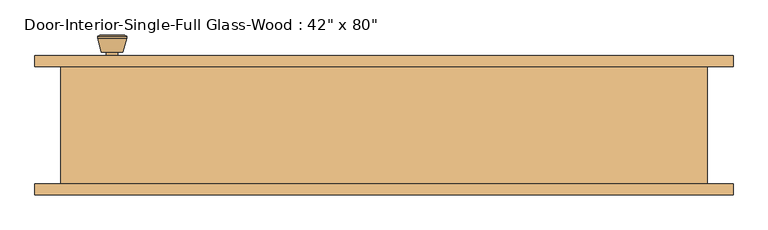
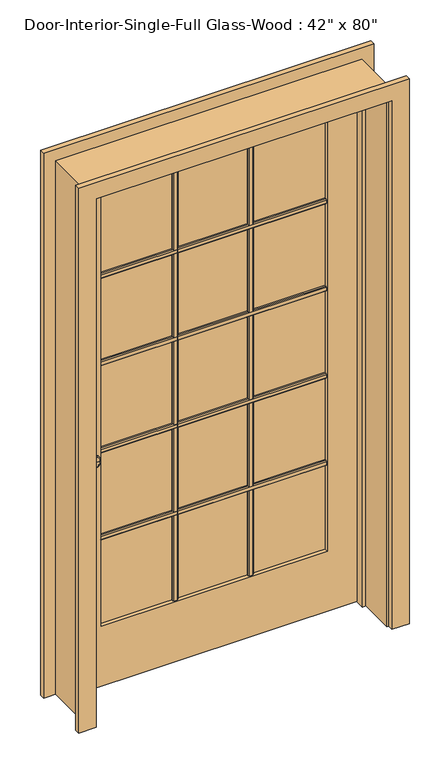
"""IFC4 building model written with IfcOpenShell, lengths in millimetres: door geometry."""

from ifc_helpers import new_model, si_unit, point, frame, frame_2d, origin, place, context, project, spatial, polyline, circle_curve, trimmed, segment, composite_curve, outline, extrude, faceted_brep, source, transform, mapped, element, save
from ifc_brep_helpers import plane_surface, cylinder_surface, revolved_surface, advanced_brep


def door_f3911013(model_context):
    return source(origin(), model_context, "Body", "SolidModel", [
        extrude(outline(polyline([(84.455, 1586.23), (90.805, 1586.23), (93.98, 1583.055), (93.98, 1570.355), (90.805, 1567.18), (84.455, 1567.18), (84.455, 1586.23)])), frame((-412.75, 0.0, 0.0), z_axis=(1.0, 0.0, 0.0), x_axis=(0.0, 1.0, 0.0)), (0.0, 0.0, 1.0), 825.5),
        extrude(outline(polyline([(84.455, 1249.9975), (90.805, 1249.9975), (93.98, 1246.8225), (93.98, 1234.1225), (90.805, 1230.9475), (84.455, 1230.9475), (84.455, 1249.9975)])), frame((-412.75, 0.0, 0.0), z_axis=(1.0, 0.0, 0.0), x_axis=(0.0, 1.0, 0.0)), (0.0, 0.0, 1.0), 825.5),
        extrude(outline(polyline([(84.455, 913.765), (90.805, 913.765), (93.98, 910.59), (93.98, 897.89), (90.805, 894.715), (84.455, 894.715), (84.455, 913.765)])), frame((-412.75, 0.0, 0.0), z_axis=(1.0, 0.0, 0.0), x_axis=(0.0, 1.0, 0.0)), (0.0, 0.0, 1.0), 825.5),
        extrude(outline(polyline([(84.455, 577.5325), (90.805, 577.5325), (93.98, 574.3575), (93.98, 561.6575), (90.805, 558.4825), (84.455, 558.4825), (84.455, 577.5325)])), frame((-412.75, 0.0, 0.0), z_axis=(1.0, 0.0, 0.0), x_axis=(0.0, 1.0, 0.0)), (0.0, 0.0, 1.0), 825.5),
        extrude(outline(polyline([(128.0583333, 84.455), (128.0583333, 90.805), (131.2333333, 93.98), (143.9333333, 93.98), (147.1083333, 90.805), (147.1083333, 84.455), (128.0583333, 84.455)])), frame((0.0, 0.0, 231.775), z_axis=(0.0, 0.0, 1.0), x_axis=(1.0, 0.0, 0.0)), (0.0, 0.0, 1.0), 1681.1625),
        extrude(outline(polyline([(-147.1083333, 84.455), (-147.1083333, 90.805), (-143.9333333, 93.98), (-131.2333333, 93.98), (-128.0583333, 90.805), (-128.0583333, 84.455), (-147.1083333, 84.455)])), frame((0.0, 0.0, 231.775), z_axis=(0.0, 0.0, 1.0), x_axis=(1.0, 0.0, 0.0)), (0.0, 0.0, 1.0), 1681.1625),
        extrude(outline(polyline([(77.47, 1586.23), (77.47, 1567.18), (71.12, 1567.18), (67.945, 1570.355), (67.945, 1583.055), (71.12, 1586.23), (77.47, 1586.23)])), frame((-412.75, 0.0, 0.0), z_axis=(1.0, 0.0, 0.0), x_axis=(0.0, 1.0, 0.0)), (0.0, 0.0, 1.0), 825.5),
        extrude(outline(polyline([(77.47, 1249.9975), (77.47, 1230.9475), (71.12, 1230.9475), (67.945, 1234.1225), (67.945, 1246.8225), (71.12, 1249.9975), (77.47, 1249.9975)])), frame((-412.75, 0.0, 0.0), z_axis=(1.0, 0.0, 0.0), x_axis=(0.0, 1.0, 0.0)), (0.0, 0.0, 1.0), 825.5),
        extrude(outline(polyline([(77.47, 913.765), (77.47, 894.715), (71.12, 894.715), (67.945, 897.89), (67.945, 910.59), (71.12, 913.765), (77.47, 913.765)])), frame((-412.75, 0.0, 0.0), z_axis=(1.0, 0.0, 0.0), x_axis=(0.0, 1.0, 0.0)), (0.0, 0.0, 1.0), 825.5),
        extrude(outline(polyline([(77.47, 577.5325), (77.47, 558.4825), (71.12, 558.4825), (67.945, 561.6575), (67.945, 574.3575), (71.12, 577.5325), (77.47, 577.5325)])), frame((-412.75, 0.0, 0.0), z_axis=(1.0, 0.0, 0.0), x_axis=(0.0, 1.0, 0.0)), (0.0, 0.0, 1.0), 825.5),
        extrude(outline(polyline([(128.0583333, 77.47), (147.1083333, 77.47), (147.1083333, 71.12), (143.9333333, 67.945), (131.2333333, 67.945), (128.0583333, 71.12), (128.0583333, 77.47)])), frame((0.0, 0.0, 231.775), z_axis=(0.0, 0.0, 1.0), x_axis=(1.0, 0.0, 0.0)), (0.0, 0.0, 1.0), 1681.1625),
        extrude(outline(polyline([(-147.1083333, 77.47), (-128.0583333, 77.47), (-128.0583333, 71.12), (-131.2333333, 67.945), (-143.9333333, 67.945), (-147.1083333, 71.12), (-147.1083333, 77.47)])), frame((0.0, 0.0, 231.775), z_axis=(0.0, 0.0, 1.0), x_axis=(1.0, 0.0, 0.0)), (0.0, 0.0, 1.0), 1681.1625),
        advanced_brep(
        [(-469.9, 57.5, 914.4), (-459.9, 57.5, 914.4), (-479.9, 57.5, 914.4), (-449.4241324, 8.5, 914.4), (-469.9, 8.5, 914.4), (-490.3758676, 8.5, 914.4), (-444.9, 10.3278681, 914.4), (-494.9, 10.3278681, 914.4), (-444.9, 13.7915463, 914.4), (-494.9, 13.7915463, 914.4), (-451.263764, 38.5, 914.4), (-488.536236, 38.5, 914.4), (-459.9, 38.5, 914.4), (-479.9, 38.5, 914.4)],
        [
            (0, 1),
            (1, 2, circle_curve(frame((-469.9, 57.5, 914.4), z_axis=(0.0, 1.0, 0.0), x_axis=(-1.0, 0.0, 0.0)), 10.0)),
            (2, 0),
            (2, 1, circle_curve(frame((-469.9, 57.5, 914.4), z_axis=(0.0, 1.0, 0.0), x_axis=(-1.0, 0.0, 0.0)), 10.0)),
            (3, 4),
            (4, 5),
            (5, 3, circle_curve(frame((-469.9, 8.5, 914.4), z_axis=(0.0, -1.0, 0.0), x_axis=(-1.0, 0.0, 0.0)), 20.4758676)),
            (3, 5, circle_curve(frame((-469.9, 8.5, 914.4), z_axis=(0.0, -1.0, 0.0), x_axis=(-1.0, 0.0, 0.0)), 20.4758676)),
            (6, 3),
            (5, 7),
            (7, 6, circle_curve(frame((-469.9, 10.3278681, 914.4), z_axis=(0.0, -1.0, 0.0), x_axis=(-1.0, 0.0, 0.0)), 25.0)),
            (6, 7, circle_curve(frame((-469.9, 10.3278681, 914.4), z_axis=(0.0, -1.0, 0.0), x_axis=(-1.0, 0.0, 0.0)), 25.0)),
            (8, 6),
            (7, 9),
            (9, 8, circle_curve(frame((-469.9, 13.7915463, 914.4), z_axis=(0.0, -1.0, 0.0), x_axis=(-1.0, 0.0, 0.0)), 25.0)),
            (8, 9, circle_curve(frame((-469.9, 13.7915463, 914.4), z_axis=(0.0, -1.0, 0.0), x_axis=(-1.0, 0.0, 0.0)), 25.0)),
            (10, 8),
            (9, 11),
            (11, 10, circle_curve(frame((-469.9, 38.5, 914.4), z_axis=(0.0, -1.0, 0.0), x_axis=(-1.0, 0.0, 0.0)), 18.636236)),
            (10, 11, circle_curve(frame((-469.9, 38.5, 914.4), z_axis=(0.0, -1.0, 0.0), x_axis=(-1.0, 0.0, 0.0)), 18.636236)),
            (12, 10),
            (11, 13),
            (13, 12, circle_curve(frame((-469.9, 38.5, 914.4), z_axis=(0.0, -1.0, 0.0), x_axis=(-1.0, 0.0, 0.0)), 10.0)),
            (12, 13, circle_curve(frame((-469.9, 38.5, 914.4), z_axis=(0.0, -1.0, 0.0), x_axis=(-1.0, 0.0, 0.0)), 10.0)),
            (1, 12),
            (13, 2),
        ],
        [
            plane_surface(frame((-469.9, 57.5, 914.4), z_axis=(0.0, 1.0, 0.0), x_axis=(-1.0, 0.0, 0.0))),
            plane_surface(frame((-469.9, 8.5, 914.4), z_axis=(0.0, -1.0, 0.0), x_axis=(-1.0, 0.0, 0.0))),
            revolved_surface(polyline([(-490.3758676, 8.5, 914.4), (-494.9, 10.3278681, 914.4)]), (-469.9, 57.5, 914.4), (0.0, 1.0, 0.0)),
            cylinder_surface(frame((-469.9, 57.5, 914.4), z_axis=(0.0, 1.0, 0.0), x_axis=(-1.0, 0.0, 0.0)), 25.0),
            revolved_surface(polyline([(-494.9, 13.7915463, 914.4), (-488.536236, 38.5, 914.4)]), (-469.9, 57.5, 914.4), (0.0, 1.0, 0.0)),
            plane_surface(frame((-469.9, 38.5, 914.4), z_axis=(0.0, 1.0, 0.0), x_axis=(-1.0, 0.0, 0.0))),
            cylinder_surface(frame((-469.9, 57.5, 914.4), z_axis=(0.0, 1.0, 0.0), x_axis=(-1.0, 0.0, 0.0)), 10.0),
        ],
        [
            (0, [[1, 2, 3]]),
            (0, [[-3, 4, -1]]),
            (1, [[5, 6, 7]]),
            (1, [[-6, -5, 8]]),
            (2, [[9, -7, 10, 11]]),
            (2, [[-10, -8, -9, 12]]),
            (3, [[13, -11, 14, 15]]),
            (3, [[-14, -12, -13, 16]]),
            (4, [[17, -15, 18, 19]]),
            (4, [[-18, -16, -17, 20]]),
            (5, [[21, -19, 22, 23]]),
            (5, [[-22, -20, -21, 24]]),
            (6, [[25, -23, 26, -2]]),
            (6, [[-26, -24, -25, -4]]),
        ],
    ),
        extrude(outline(composite_curve([segment(trimmed(circle_curve(frame_2d((914.4, -469.9)), 30.0), [point((914.4, -499.9))], [point((914.4, -439.9))], False, "CARTESIAN"), True, "CONTINUOUS"), segment(trimmed(circle_curve(frame_2d((914.4, -469.9)), 30.0), [point((914.4, -439.9))], [point((914.4, -499.9))], False, "CARTESIAN"), True, "CONTINUOUS")], self_intersect=False)), frame((0.0, 57.5, 0.0), z_axis=(0.0, 1.0, 0.0), x_axis=(0.0, 0.0, 1.0)), (0.0, 0.0, 1.0), 6.0),
        advanced_brep(
        [(-469.9, 104.425, 914.4), (-479.9, 104.425, 914.4), (-459.9, 104.425, 914.4), (-449.4241324, 153.425, 914.4), (-490.3758676, 153.425, 914.4), (-469.9, 153.425, 914.4), (-444.9, 151.5971319, 914.4), (-494.9, 151.5971319, 914.4), (-444.9, 148.1334537, 914.4), (-494.9, 148.1334537, 914.4), (-451.263764, 123.425, 914.4), (-488.536236, 123.425, 914.4), (-459.9, 123.425, 914.4), (-479.9, 123.425, 914.4)],
        [
            (0, 1),
            (1, 2, circle_curve(frame((-469.9, 104.425, 914.4), z_axis=(0.0, -1.0, 0.0), x_axis=(-1.0, 0.0, 0.0)), 10.0)),
            (2, 0),
            (2, 1, circle_curve(frame((-469.9, 104.425, 914.4), z_axis=(0.0, -1.0, 0.0), x_axis=(-1.0, 0.0, 0.0)), 10.0)),
            (3, 4, circle_curve(frame((-469.9, 153.425, 914.4), z_axis=(0.0, 1.0, 0.0), x_axis=(-1.0, 0.0, 0.0)), 20.4758676)),
            (4, 5),
            (5, 3),
            (4, 3, circle_curve(frame((-469.9, 153.425, 914.4), z_axis=(0.0, 1.0, 0.0), x_axis=(-1.0, 0.0, 0.0)), 20.4758676)),
            (6, 7, circle_curve(frame((-469.9, 151.5971319, 914.4), z_axis=(0.0, 1.0, 0.0), x_axis=(-1.0, 0.0, 0.0)), 25.0)),
            (7, 4),
            (3, 6),
            (7, 6, circle_curve(frame((-469.9, 151.5971319, 914.4), z_axis=(0.0, 1.0, 0.0), x_axis=(-1.0, 0.0, 0.0)), 25.0)),
            (8, 9, circle_curve(frame((-469.9, 148.1334537, 914.4), z_axis=(0.0, 1.0, 0.0), x_axis=(-1.0, 0.0, 0.0)), 25.0)),
            (9, 7),
            (6, 8),
            (9, 8, circle_curve(frame((-469.9, 148.1334537, 914.4), z_axis=(0.0, 1.0, 0.0), x_axis=(-1.0, 0.0, 0.0)), 25.0)),
            (10, 11, circle_curve(frame((-469.9, 123.425, 914.4), z_axis=(0.0, 1.0, 0.0), x_axis=(-1.0, 0.0, 0.0)), 18.636236)),
            (11, 9),
            (8, 10),
            (11, 10, circle_curve(frame((-469.9, 123.425, 914.4), z_axis=(0.0, 1.0, 0.0), x_axis=(-1.0, 0.0, 0.0)), 18.636236)),
            (12, 13, circle_curve(frame((-469.9, 123.425, 914.4), z_axis=(0.0, 1.0, 0.0), x_axis=(-1.0, 0.0, 0.0)), 10.0)),
            (13, 11),
            (10, 12),
            (13, 12, circle_curve(frame((-469.9, 123.425, 914.4), z_axis=(0.0, 1.0, 0.0), x_axis=(-1.0, 0.0, 0.0)), 10.0)),
            (1, 13),
            (12, 2),
        ],
        [
            plane_surface(frame((-469.9, 104.425, 914.4), z_axis=(0.0, -1.0, 0.0), x_axis=(-1.0, 0.0, 0.0))),
            plane_surface(frame((-469.9, 153.425, 914.4), z_axis=(0.0, 1.0, 0.0), x_axis=(-1.0, 0.0, 0.0))),
            revolved_surface(polyline([(-490.3758676, 153.425, 914.4), (-494.9, 151.5971319, 914.4)]), (-469.9, 104.425, 914.4), (0.0, -1.0, 0.0)),
            cylinder_surface(frame((-469.9, 104.425, 914.4), z_axis=(0.0, -1.0, 0.0), x_axis=(-1.0, 0.0, 0.0)), 25.0),
            revolved_surface(polyline([(-494.9, 148.1334537, 914.4), (-488.536236, 123.425, 914.4)]), (-469.9, 104.425, 914.4), (0.0, -1.0, 0.0)),
            plane_surface(frame((-469.9, 123.425, 914.4), z_axis=(0.0, -1.0, 0.0), x_axis=(-1.0, 0.0, 0.0))),
            cylinder_surface(frame((-469.9, 104.425, 914.4), z_axis=(0.0, -1.0, 0.0), x_axis=(-1.0, 0.0, 0.0)), 10.0),
        ],
        [
            (0, [[1, 2, 3]]),
            (0, [[-3, 4, -1]]),
            (1, [[5, 6, 7]]),
            (1, [[8, -7, -6]]),
            (2, [[9, 10, -5, 11]]),
            (2, [[12, -11, -8, -10]]),
            (3, [[13, 14, -9, 15]]),
            (3, [[16, -15, -12, -14]]),
            (4, [[17, 18, -13, 19]]),
            (4, [[20, -19, -16, -18]]),
            (5, [[21, 22, -17, 23]]),
            (5, [[24, -23, -20, -22]]),
            (6, [[-2, 25, -21, 26]]),
            (6, [[-4, -26, -24, -25]]),
        ],
    ),
        extrude(outline(composite_curve([segment(trimmed(circle_curve(frame_2d((914.4, -469.9)), 30.0), [point((914.4, -499.9))], [point((914.4, -439.9))], False, "CARTESIAN"), True, "CONTINUOUS"), segment(trimmed(circle_curve(frame_2d((914.4, -469.9)), 30.0), [point((914.4, -439.9))], [point((914.4, -499.9))], False, "CARTESIAN"), True, "CONTINUOUS")], self_intersect=False)), frame((0.0, 98.425, 0.0), z_axis=(0.0, 1.0, 0.0), x_axis=(0.0, 0.0, 1.0)), (0.0, 0.0, 1.0), 6.0),
        extrude(outline(polyline([(2032.0, -533.4), (0.0, -533.4), (0.0, 533.4), (2032.0, 533.4), (2032.0, -533.4)]), holes=[polyline([(1912.9375, -412.75), (1912.9375, 412.75), (231.775, 412.75), (231.775, -412.75), (1912.9375, -412.75)])]), frame((0.0, 63.5, 0.0), z_axis=(0.0, 1.0, 0.0), x_axis=(0.0, 0.0, 1.0)), (0.0, 0.0, 1.0), 34.925),
        faceted_brep([(558.8, 98.425, 0.0), (558.8, -104.775, 0.0), (533.4, -104.775, 0.0), (533.4, 28.575, 0.0), (520.7, 28.575, 0.0), (520.7, 63.5, 0.0), (533.4, 63.5, 0.0), (533.4, 98.425, 0.0), (558.8, 98.425, 2057.4), (558.8, -104.775, 2057.4), (-558.8, -104.775, 2057.4), (-558.8, -104.775, 0.0), (-533.4, -104.775, 0.0), (-533.4, -104.775, 2032.0), (533.4, -104.775, 2032.0), (533.4, 28.575, 2032.0), (-533.4, 28.575, 2032.0), (-533.4, 28.575, 0.0), (-520.7, 28.575, 0.0), (-520.7, 28.575, 2019.3), (520.7, 28.575, 2019.3), (520.7, 63.5, 2019.3), (-520.7, 63.5, 2019.3), (-520.7, 63.5, 0.0), (-533.4, 63.5, 0.0), (-533.4, 63.5, 2032.0), (533.4, 63.5, 2032.0), (533.4, 98.425, 2032.0), (-533.4, 98.425, 2032.0), (-533.4, 98.425, 0.0), (-558.8, 98.425, 0.0), (-558.8, 98.425, 2057.4)], [[[0, 1, 2, 3, 4, 5, 6, 7]], [[1, 0, 8, 9]], [[2, 1, 9, 10, 11, 12, 13, 14]], [[3, 2, 14, 15]], [[4, 3, 15, 16, 17, 18, 19, 20]], [[5, 4, 20, 21]], [[6, 5, 21, 22, 23, 24, 25, 26]], [[7, 6, 26, 27]], [[0, 7, 27, 28, 29, 30, 31, 8]], [[9, 8, 31, 10]], [[15, 14, 13, 16]], [[21, 20, 19, 22]], [[27, 26, 25, 28]], [[30, 29, 24, 23, 18, 17, 12, 11]], [[10, 31, 30, 11]], [[16, 13, 12, 17]], [[22, 19, 18, 23]], [[28, 25, 24, 29]]]),
        extrude(outline(polyline([(412.75, 77.47), (-412.75, 77.47), (-412.75, 84.455), (412.75, 84.455), (412.75, 77.47)])), frame((0.0, 0.0, 231.775), z_axis=(0.0, 0.0, 1.0), x_axis=(1.0, 0.0, 0.0)), (0.0, 0.0, 1.0), 1681.1625),
        extrude(outline(polyline([(0.0, 539.75), (0.0, 603.25), (2101.85, 603.25), (2101.85, -603.25), (0.0, -603.25), (0.0, -539.75), (2038.35, -539.75), (2038.35, 539.75), (0.0, 539.75)])), frame((0.0, -123.825, 0.0), z_axis=(0.0, 1.0, 0.0), x_axis=(0.0, 0.0, 1.0)), (0.0, 0.0, 1.0), 19.05),
        extrude(outline(polyline([(0.0, 539.75), (0.0, 603.25), (2101.85, 603.25), (2101.85, -603.25), (0.0, -603.25), (0.0, -539.75), (2038.35, -539.75), (2038.35, 539.75), (0.0, 539.75)])), frame((0.0, 98.425, 0.0), z_axis=(0.0, 1.0, 0.0), x_axis=(0.0, 0.0, 1.0)), (0.0, 0.0, 1.0), 19.05),
    ])


if __name__ == "__main__":
    model = new_model("IFC4")
    model_context = context("Model", 3, world=origin())
    ifc_project = project(units=[si_unit("LENGTHUNIT", "METRE", prefix="MILLI")], contexts=[model_context])
    site = spatial("IfcSite", under=ifc_project)
    building = spatial("IfcBuilding", under=site)
    placement = place(None, origin())
    door_shape = door_f3911013(model_context)
    element("IfcDoor", 1, ObjectType="Door-Interior-Single-Full Glass-Wood : 42\" x 80\"", at=placement, inside=building, context=model_context, shape_type="MappedRepresentation", body=[
        mapped(door_shape, transform((0.0, 0.0, 0.0), x_axis=(1.0, 0.0, 0.0), y_axis=(0.0, 1.0, 0.0), z_axis=(0.0, 0.0, 1.0))),
    ])
    save(model, "model.ifc")

# Revit data of these elements
# Type "Door-Interior-Single-Full Glass-Wood : 42\" x 80\""
#   Type Mark = "10"
#   Assembly Code = "C1020300"
#   Analytic Construction = "Wood frame with single clear glass"
#   Top Rail = 0' - 4 11/16"
#   Thickness = 0' - 1 3/8"
#   Thermal Resistance (R) = 1.0102 (h·ft²·°F)/BTU
#   Swing Angle [instance default] = 90.00°
#   Stiles = 0' - 4 3/4"
#   Rough Width = 3' - 8"
#   Rough Height = 6' - 9"
#   Height = 6' - 8"
#   Width = 3' - 6"
#   Heat Transfer Coefficient (U) = 0.9900 BTU/(h·ft²·°F)
#   Bottom Rail = 0' - 9 1/8"
#   Show Grill [instance default] = yes
#   Trim Material = Cherry
#   Panel Material = Cherry
#   Frame Material = Cherry
#   Door Handle Material = Aluminum
#   Visual Light Transmittance = 0
#   Solar Heat Gain Coefficient = 0
#   Wall Closure = (empty or 0)
#   Function = (empty or 0)
# Element 1 (IfcDoor, "Door-Interior-Single-Full Glass-Wood : 42\" x 80\"")
#   Materials on its faces: "Cherry", "Aluminum", "Glass"
# Materials
#   "Cherry": class "Wood", colour RGB 226 177 128, transparency 0, Description = "Prunus Serotina", Cost = 0
#   "Aluminum": class "Metal", colour RGB 247 247 247, transparency 0, Description = "Aluminum 6061", Cost = 0
#   "Glass": class "Glass", colour RGB 0 128 192, transparency 0.75, Description = "Soda Lime Glass", Cost = 0
